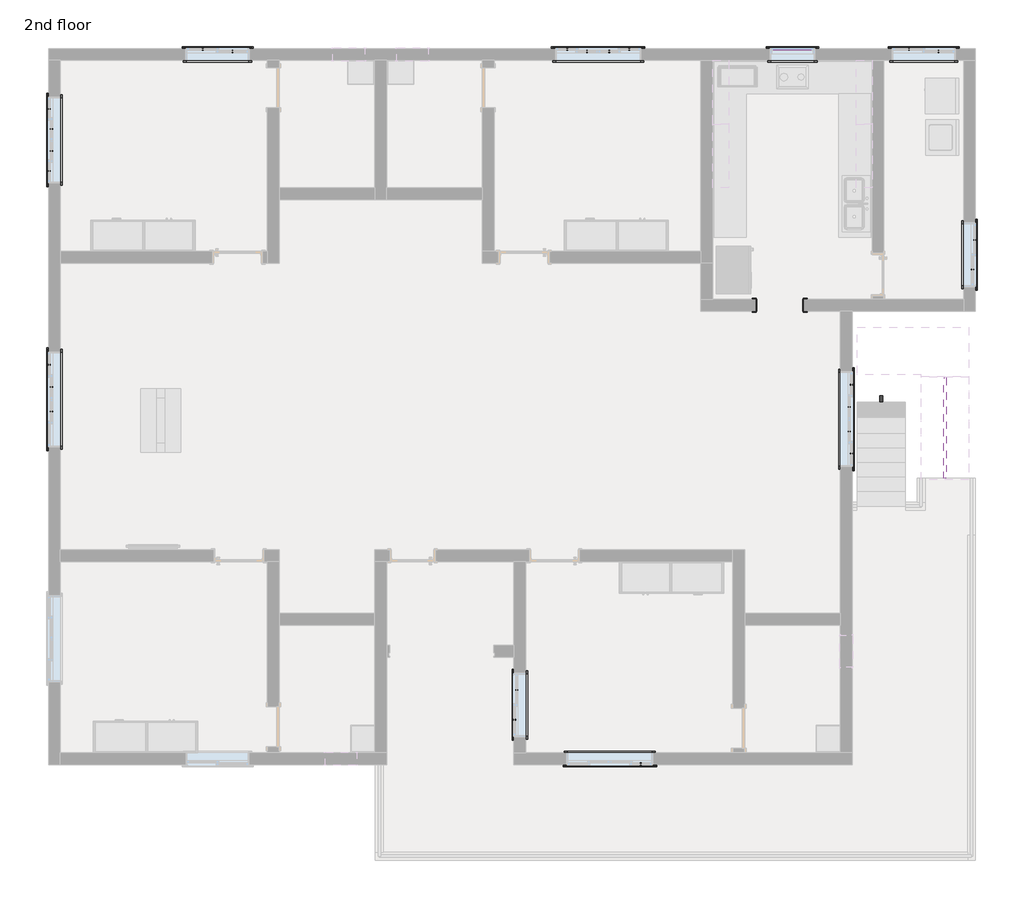
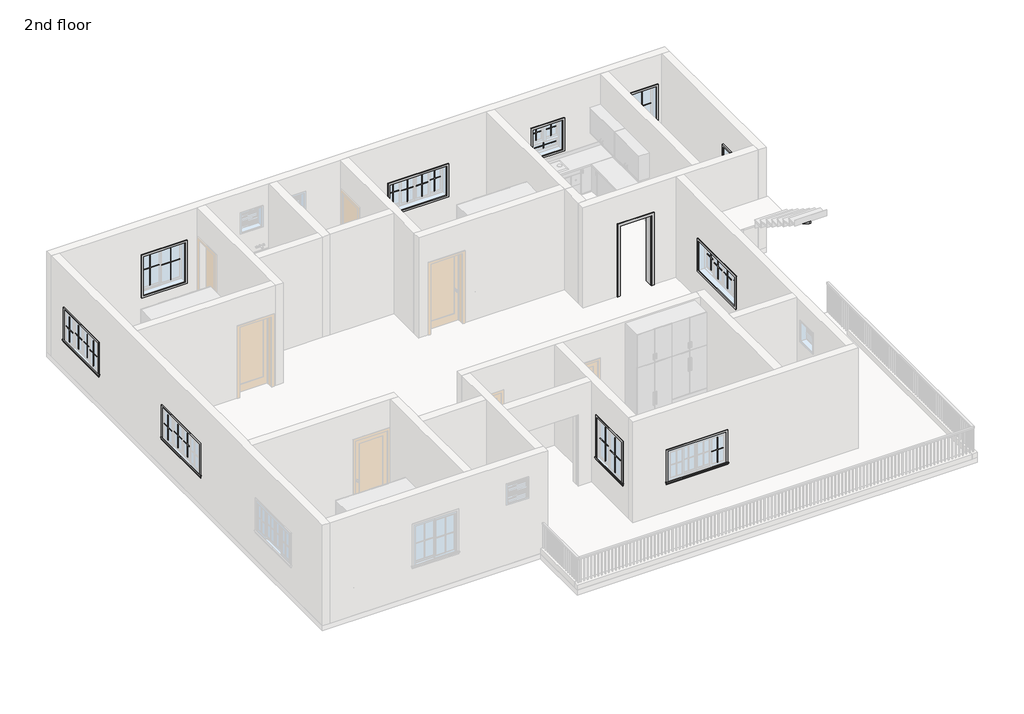
# One storey, part 4 of 4: 48 proxies, 2 members.
"""IFC4 building model written with IfcOpenShell, lengths in millimetres."""

from ifc_helpers import new_model, si_unit, frame, origin, place, context, project, spatial, polyline, outline, extrude, transform, mapped, element, save
from components import muntin_pattern_2x2_muntin_pattern_2x2_6186d23a, muntin_pattern_2x2_muntin_pattern_2x2_31a16349, muntin_pattern_2x2_muntin_pattern_2x2_cf37b409, muntin_pattern_2x2_muntin_pattern_2x2_78ce0566, muntin_pattern_2x2_muntin_pattern_2x2_27bf4e5b, muntin_pattern_2x2_muntin_pattern_2x2_8320156c, proxy_e9bf662a, trim_window_exterior_flat_with_sill_c3f87112, trim_window_exterior_flat_with_sill_3c945769, trim_window_exterior_flat_with_sill_7cfdd449, trim_window_exterior_flat_with_sill_41619996, trim_window_interior_flat_picture_frame_1c33fa8a, trim_window_interior_flat_picture_frame_0edfbaa2, trim_window_interior_flat_picture_frame_f1e0b15b, trim_window_interior_flat_picture_frame_51c85655

model = new_model("IFC4")

# Units and contexts
model_context = context("Model", 3, world=origin())
ifc_project = project(units=[si_unit("LENGTHUNIT", "METRE", prefix="MILLI")], contexts=[model_context])

# Site, building, storey
site = spatial("IfcSite", under=ifc_project)
building = spatial("IfcBuilding", under=site)
storey = spatial("IfcBuildingStorey", under=building, Name="2nd floor", Elevation=7010.4)

# Proxies
placement = place(None, origin())
muntin_pattern_2x2_muntin_pattern_2x2_shape = muntin_pattern_2x2_muntin_pattern_2x2_6186d23a(model_context)
element("IfcBuildingElementProxy", 1, Name="Muntin Pattern_2x2 : Muntin Pattern_2x2", ObjectType="Muntin Pattern_2x2 : Muntin Pattern_2x2", at=placement, inside=storey, context=model_context, shape_type="MappedRepresentation", body=[
    mapped(muntin_pattern_2x2_muntin_pattern_2x2_shape, transform((1905.0010838, 7064.4410813, 8007.35), x_axis=(1.0, 0.0, 0.0), y_axis=(0.0, 1.0, 0.0), z_axis=(0.0, 0.0, 1.0))),
])
element("IfcBuildingElementProxy", 2, Name="Muntin Pattern_2x2 : Muntin Pattern_2x2", ObjectType="Muntin Pattern_2x2 : Muntin Pattern_2x2", at=placement, inside=storey, context=model_context, shape_type="MappedRepresentation", body=[
    mapped(muntin_pattern_2x2_muntin_pattern_2x2_shape, transform((2286.0010838, 7019.9910813, 8007.35), x_axis=(1.0, 0.0, 0.0), y_axis=(0.0, 1.0, 0.0), z_axis=(0.0, 0.0, 1.0))),
])
element("IfcBuildingElementProxy", 3, Name="Muntin Pattern_2x2 : Muntin Pattern_2x2", ObjectType="Muntin Pattern_2x2 : Muntin Pattern_2x2", at=placement, inside=storey, context=model_context, shape_type="MappedRepresentation", body=[
    mapped(muntin_pattern_2x2_muntin_pattern_2x2_shape, transform((2711.4510838, 7019.9910813, 8007.35), x_axis=(1.0, 0.0, 0.0), y_axis=(0.0, 1.0, 0.0), z_axis=(0.0, 0.0, 1.0))),
])
element("IfcBuildingElementProxy", 4, Name="Muntin Pattern_2x2 : Muntin Pattern_2x2", ObjectType="Muntin Pattern_2x2 : Muntin Pattern_2x2", at=placement, inside=storey, context=model_context, shape_type="MappedRepresentation", body=[
    mapped(muntin_pattern_2x2_muntin_pattern_2x2_shape, transform((3092.4510838, 7064.4410813, 8007.35), x_axis=(1.0, 0.0, 0.0), y_axis=(0.0, 1.0, 0.0), z_axis=(0.0, 0.0, 1.0))),
])
element("IfcBuildingElementProxy", 5, Name="Muntin Pattern_2x2 : Muntin Pattern_2x2", ObjectType="Muntin Pattern_2x2 : Muntin Pattern_2x2", at=placement, inside=storey, context=model_context, shape_type="MappedRepresentation", body=[
    mapped(muntin_pattern_2x2_muntin_pattern_2x2_shape, transform((3314.7010838, -6632.5089187, 8007.35), x_axis=(-1.0, 0.0, 0.0), y_axis=(0.0, -1.0, 0.0), z_axis=(0.0, 0.0, 1.0))),
])
element("IfcBuildingElementProxy", 6, Name="Muntin Pattern_2x2 : Muntin Pattern_2x2", ObjectType="Muntin Pattern_2x2 : Muntin Pattern_2x2", at=placement, inside=storey, context=model_context, shape_type="MappedRepresentation", body=[
    mapped(muntin_pattern_2x2_muntin_pattern_2x2_shape, transform((-8020.0489162, 4727.6410813, 8007.35), x_axis=(0.0, 1.0, 0.0), y_axis=(-1.0, 0.0, 0.0), z_axis=(0.0, 0.0, 1.0))),
])
element("IfcBuildingElementProxy", 7, Name="Muntin Pattern_2x2 : Muntin Pattern_2x2", ObjectType="Muntin Pattern_2x2 : Muntin Pattern_2x2", at=placement, inside=storey, context=model_context, shape_type="MappedRepresentation", body=[
    mapped(muntin_pattern_2x2_muntin_pattern_2x2_shape, transform((-7975.5989162, 5108.6410813, 8007.35), x_axis=(0.0, 1.0, 0.0), y_axis=(-1.0, 0.0, 0.0), z_axis=(0.0, 0.0, 1.0))),
])
element("IfcBuildingElementProxy", 8, Name="Muntin Pattern_2x2 : Muntin Pattern_2x2", ObjectType="Muntin Pattern_2x2 : Muntin Pattern_2x2", at=placement, inside=storey, context=model_context, shape_type="MappedRepresentation", body=[
    mapped(muntin_pattern_2x2_muntin_pattern_2x2_shape, transform((-7975.5989162, 5534.0910813, 8007.35), x_axis=(0.0, 1.0, 0.0), y_axis=(-1.0, 0.0, 0.0), z_axis=(0.0, 0.0, 1.0))),
])
element("IfcBuildingElementProxy", 9, Name="Muntin Pattern_2x2 : Muntin Pattern_2x2", ObjectType="Muntin Pattern_2x2 : Muntin Pattern_2x2", at=placement, inside=storey, context=model_context, shape_type="MappedRepresentation", body=[
    mapped(muntin_pattern_2x2_muntin_pattern_2x2_shape, transform((-8020.0489162, 5915.0910813, 8007.35), x_axis=(0.0, 1.0, 0.0), y_axis=(-1.0, 0.0, 0.0), z_axis=(0.0, 0.0, 1.0))),
])
muntin_pattern_2x2_muntin_pattern_2x2_2_shape = muntin_pattern_2x2_muntin_pattern_2x2_31a16349(model_context)
element("IfcBuildingElementProxy", 10, Name="Muntin Pattern_2x2 : Muntin Pattern_2x2", ObjectType="Muntin Pattern_2x2 : Muntin Pattern_2x2", at=placement, inside=storey, context=model_context, shape_type="MappedRepresentation", body=[
    mapped(muntin_pattern_2x2_muntin_pattern_2x2_2_shape, transform((-7975.5989162, 120.7160813, 8007.35), x_axis=(0.0, 1.0, 0.0), y_axis=(-1.0, 0.0, 0.0), z_axis=(0.0, 0.0, 1.0))),
])
element("IfcBuildingElementProxy", 11, Name="Muntin Pattern_2x2 : Muntin Pattern_2x2", ObjectType="Muntin Pattern_2x2 : Muntin Pattern_2x2", at=placement, inside=storey, context=model_context, shape_type="MappedRepresentation", body=[
    mapped(muntin_pattern_2x2_muntin_pattern_2x2_2_shape, transform((-7975.5989162, 590.6160813, 8007.35), x_axis=(0.0, 1.0, 0.0), y_axis=(-1.0, 0.0, 0.0), z_axis=(0.0, 0.0, 1.0))),
])
element("IfcBuildingElementProxy", 12, Name="Muntin Pattern_2x2 : Muntin Pattern_2x2", ObjectType="Muntin Pattern_2x2 : Muntin Pattern_2x2", at=placement, inside=storey, context=model_context, shape_type="MappedRepresentation", body=[
    mapped(muntin_pattern_2x2_muntin_pattern_2x2_2_shape, transform((-8020.0489162, 1016.0660813, 8007.35), x_axis=(0.0, 1.0, 0.0), y_axis=(-1.0, 0.0, 0.0), z_axis=(0.0, 0.0, 1.0))),
])
element("IfcBuildingElementProxy", 13, Name="Muntin Pattern_2x2 : Muntin Pattern_2x2", ObjectType="Muntin Pattern_2x2 : Muntin Pattern_2x2", at=placement, inside=storey, context=model_context, shape_type="MappedRepresentation", body=[
    mapped(muntin_pattern_2x2_muntin_pattern_2x2_2_shape, transform((7353.3010838, 635.0660813, 8007.35), x_axis=(0.0, -1.0, 0.0), y_axis=(1.0, 0.0, 0.0), z_axis=(0.0, 0.0, 1.0))),
])
element("IfcBuildingElementProxy", 14, Name="Muntin Pattern_2x2 : Muntin Pattern_2x2", ObjectType="Muntin Pattern_2x2 : Muntin Pattern_2x2", at=placement, inside=storey, context=model_context, shape_type="MappedRepresentation", body=[
    mapped(muntin_pattern_2x2_muntin_pattern_2x2_2_shape, transform((7308.8510838, 209.6160813, 8007.35), x_axis=(0.0, -1.0, 0.0), y_axis=(1.0, 0.0, 0.0), z_axis=(0.0, 0.0, 1.0))),
])
element("IfcBuildingElementProxy", 15, Name="Muntin Pattern_2x2 : Muntin Pattern_2x2", ObjectType="Muntin Pattern_2x2 : Muntin Pattern_2x2", at=placement, inside=storey, context=model_context, shape_type="MappedRepresentation", body=[
    mapped(muntin_pattern_2x2_muntin_pattern_2x2_2_shape, transform((7308.8510838, -260.2839187, 8007.35), x_axis=(0.0, -1.0, 0.0), y_axis=(1.0, 0.0, 0.0), z_axis=(0.0, 0.0, 1.0))),
])
element("IfcBuildingElementProxy", 16, Name="Muntin Pattern_2x2 : Muntin Pattern_2x2", ObjectType="Muntin Pattern_2x2 : Muntin Pattern_2x2", at=placement, inside=storey, context=model_context, shape_type="MappedRepresentation", body=[
    mapped(muntin_pattern_2x2_muntin_pattern_2x2_2_shape, transform((7353.3010838, -685.7339187, 8007.35), x_axis=(0.0, -1.0, 0.0), y_axis=(1.0, 0.0, 0.0), z_axis=(0.0, 0.0, 1.0))),
])
muntin_pattern_2x2_muntin_pattern_2x2_3_shape = muntin_pattern_2x2_muntin_pattern_2x2_cf37b409(model_context)
element("IfcBuildingElementProxy", 17, Name="Muntin Pattern_2x2 : Muntin Pattern_2x2", ObjectType="Muntin Pattern_2x2 : Muntin Pattern_2x2", at=placement, inside=storey, context=model_context, shape_type="MappedRepresentation", body=[
    mapped(muntin_pattern_2x2_muntin_pattern_2x2_3_shape, transform((939.8010838, -5214.8714187, 8007.35), x_axis=(0.0, 1.0, 0.0), y_axis=(-1.0, 0.0, 0.0), z_axis=(0.0, 0.0, 1.0))),
])
element("IfcBuildingElementProxy", 18, Name="Muntin Pattern_2x2 : Muntin Pattern_2x2", ObjectType="Muntin Pattern_2x2 : Muntin Pattern_2x2", at=placement, inside=storey, context=model_context, shape_type="MappedRepresentation", body=[
    mapped(muntin_pattern_2x2_muntin_pattern_2x2_3_shape, transform((895.3510838, -5783.1964187, 8007.35), x_axis=(0.0, 1.0, 0.0), y_axis=(-1.0, 0.0, 0.0), z_axis=(0.0, 0.0, 1.0))),
])
element("IfcBuildingElementProxy", 19, Name="Muntin Pattern_2x2 : Muntin Pattern_2x2", ObjectType="Muntin Pattern_2x2 : Muntin Pattern_2x2", at=placement, inside=storey, context=model_context, shape_type="MappedRepresentation", body=[
    mapped(muntin_pattern_2x2_muntin_pattern_2x2_3_shape, transform((9018.5885838, 7019.9910813, 8007.35), x_axis=(1.0, 0.0, 0.0), y_axis=(0.0, 1.0, 0.0), z_axis=(0.0, 0.0, 1.0))),
])
element("IfcBuildingElementProxy", 20, Name="Muntin Pattern_2x2 : Muntin Pattern_2x2", ObjectType="Muntin Pattern_2x2 : Muntin Pattern_2x2", at=placement, inside=storey, context=model_context, shape_type="MappedRepresentation", body=[
    mapped(muntin_pattern_2x2_muntin_pattern_2x2_3_shape, transform((8450.2635838, 7064.4410813, 8007.35), x_axis=(1.0, 0.0, 0.0), y_axis=(0.0, 1.0, 0.0), z_axis=(0.0, 0.0, 1.0))),
])
element("IfcBuildingElementProxy", 21, Name="Muntin Pattern_2x2 : Muntin Pattern_2x2", ObjectType="Muntin Pattern_2x2 : Muntin Pattern_2x2", at=placement, inside=storey, context=model_context, shape_type="MappedRepresentation", body=[
    mapped(muntin_pattern_2x2_muntin_pattern_2x2_3_shape, transform((9671.0510838, 2840.1035813, 8007.35), x_axis=(0.0, -1.0, 0.0), y_axis=(1.0, 0.0, 0.0), z_axis=(0.0, 0.0, 1.0))),
])
element("IfcBuildingElementProxy", 22, Name="Muntin Pattern_2x2 : Muntin Pattern_2x2", ObjectType="Muntin Pattern_2x2 : Muntin Pattern_2x2", at=placement, inside=storey, context=model_context, shape_type="MappedRepresentation", body=[
    mapped(muntin_pattern_2x2_muntin_pattern_2x2_3_shape, transform((9715.5010838, 3408.4285813, 8007.35), x_axis=(0.0, -1.0, 0.0), y_axis=(1.0, 0.0, 0.0), z_axis=(0.0, 0.0, 1.0))),
])
element("IfcBuildingElementProxy", 23, Name="Muntin Pattern_2x2 : Muntin Pattern_2x2", ObjectType="Muntin Pattern_2x2 : Muntin Pattern_2x2", at=placement, inside=storey, context=model_context, shape_type="MappedRepresentation", body=[
    mapped(muntin_pattern_2x2_muntin_pattern_2x2_3_shape, transform((-4506.9114162, 7019.9910813, 8007.35), x_axis=(1.0, 0.0, 0.0), y_axis=(0.0, 1.0, 0.0), z_axis=(0.0, 0.0, 1.0))),
])
element("IfcBuildingElementProxy", 24, Name="Muntin Pattern_2x2 : Muntin Pattern_2x2", ObjectType="Muntin Pattern_2x2 : Muntin Pattern_2x2", at=placement, inside=storey, context=model_context, shape_type="MappedRepresentation", body=[
    mapped(muntin_pattern_2x2_muntin_pattern_2x2_3_shape, transform((-5075.2364162, 7064.4410813, 8007.35), x_axis=(1.0, 0.0, 0.0), y_axis=(0.0, 1.0, 0.0), z_axis=(0.0, 0.0, 1.0))),
])
muntin_pattern_2x2_muntin_pattern_2x2_4_shape = muntin_pattern_2x2_muntin_pattern_2x2_78ce0566(model_context)
element("IfcBuildingElementProxy", 25, Name="Muntin Pattern_2x2 : Muntin Pattern_2x2", ObjectType="Muntin Pattern_2x2 : Muntin Pattern_2x2", at=placement, inside=storey, context=model_context, shape_type="MappedRepresentation", body=[
    mapped(muntin_pattern_2x2_muntin_pattern_2x2_4_shape, transform((6005.5135838, 7064.4410813, 8528.05), x_axis=(1.0, 0.0, 0.0), y_axis=(0.0, 1.0, 0.0), z_axis=(0.0, 0.0, 1.0))),
])
muntin_pattern_2x2_muntin_pattern_2x2_5_shape = muntin_pattern_2x2_muntin_pattern_2x2_27bf4e5b(model_context)
element("IfcBuildingElementProxy", 26, Name="Muntin Pattern_2x2 : Muntin Pattern_2x2", ObjectType="Muntin Pattern_2x2 : Muntin Pattern_2x2", at=placement, inside=storey, context=model_context, shape_type="MappedRepresentation", body=[
    mapped(muntin_pattern_2x2_muntin_pattern_2x2_5_shape, transform((6434.1385838, 7064.4410813, 8528.05), x_axis=(-1.0, 0.0, 0.0), y_axis=(0.0, -1.0, 0.0), z_axis=(0.0, 0.0, 1.0))),
])
muntin_pattern_2x2_muntin_pattern_2x2_6_shape = muntin_pattern_2x2_muntin_pattern_2x2_8320156c(model_context)
element("IfcBuildingElementProxy", 27, Name="Muntin Pattern_2x2 : Muntin Pattern_2x2", ObjectType="Muntin Pattern_2x2 : Muntin Pattern_2x2", at=placement, inside=storey, context=model_context, shape_type="MappedRepresentation", body=[
    mapped(muntin_pattern_2x2_muntin_pattern_2x2_6_shape, transform((6219.8260838, 7064.4410813, 8223.25), x_axis=(-1.0, 0.0, 0.0), y_axis=(0.0, -1.0, 0.0), z_axis=(0.0, 0.0, 1.0))),
])
proxy_shape = proxy_e9bf662a(model_context)
element("IfcBuildingElementProxy", 28, Name="Passage Opening-Cased : 36\" x 84\"", ObjectType="Passage Opening-Cased : 36\" x 84\"", at=placement, inside=storey, context=model_context, shape_type="MappedRepresentation", body=[
    mapped(proxy_shape, transform((5970.337427, 2159.0660813, 7010.4), x_axis=(-1.0, 0.0, 0.0), y_axis=(0.0, -1.0, 0.0), z_axis=(0.0, 0.0, 1.0))),
])
trim_window_exterior_flat_with_sill_shape = trim_window_exterior_flat_with_sill_c3f87112(model_context)
element("IfcBuildingElementProxy", 29, Name="Trim-Window-Exterior-Flat : with Sill", ObjectType="Trim-Window-Exterior-Flat : with Sill", at=placement, inside=storey, context=model_context, shape_type="MappedRepresentation", body=[
    mapped(trim_window_exterior_flat_with_sill_shape, transform((2498.7260838, 7073.9660813, 8839.2), x_axis=(-1.0, 0.0, 0.0), y_axis=(0.0, 0.0, 1.0), z_axis=(0.0, 1.0, 0.0))),
])
element("IfcBuildingElementProxy", 30, Name="Trim-Window-Exterior-Flat : with Sill", ObjectType="Trim-Window-Exterior-Flat : with Sill", at=placement, inside=storey, context=model_context, shape_type="MappedRepresentation", body=[
    mapped(trim_window_exterior_flat_with_sill_shape, transform((2720.9760838, -6642.0339187, 8839.2), x_axis=(1.0, 0.0, 0.0), y_axis=(0.0, 0.0, 1.0), z_axis=(0.0, -1.0, 0.0))),
])
element("IfcBuildingElementProxy", 31, Name="Trim-Window-Exterior-Flat : with Sill", ObjectType="Trim-Window-Exterior-Flat : with Sill", at=placement, inside=storey, context=model_context, shape_type="MappedRepresentation", body=[
    mapped(trim_window_exterior_flat_with_sill_shape, transform((-8029.5739162, 5321.3660813, 8839.2), x_axis=(0.0, -1.0, 0.0), y_axis=(0.0, 0.0, 1.0), z_axis=(-1.0, 0.0, 0.0))),
])
trim_window_exterior_flat_with_sill_2_shape = trim_window_exterior_flat_with_sill_3c945769(model_context)
element("IfcBuildingElementProxy", 32, Name="Trim-Window-Exterior-Flat : with Sill", ObjectType="Trim-Window-Exterior-Flat : with Sill", at=placement, inside=storey, context=model_context, shape_type="MappedRepresentation", body=[
    mapped(trim_window_exterior_flat_with_sill_2_shape, transform((-8029.5739162, 355.6660813, 8839.2), x_axis=(0.0, -1.0, 0.0), y_axis=(0.0, 0.0, 1.0), z_axis=(-1.0, 0.0, 0.0))),
])
element("IfcBuildingElementProxy", 33, Name="Trim-Window-Exterior-Flat : with Sill", ObjectType="Trim-Window-Exterior-Flat : with Sill", at=placement, inside=storey, context=model_context, shape_type="MappedRepresentation", body=[
    mapped(trim_window_exterior_flat_with_sill_2_shape, transform((7362.8260838, -25.3339187, 8839.2), x_axis=(0.0, 1.0, 0.0), y_axis=(0.0, 0.0, 1.0), z_axis=(1.0, 0.0, 0.0))),
])
trim_window_exterior_flat_with_sill_3_shape = trim_window_exterior_flat_with_sill_7cfdd449(model_context)
element("IfcBuildingElementProxy", 34, Name="Trim-Window-Exterior-Flat : with Sill", ObjectType="Trim-Window-Exterior-Flat : with Sill", at=placement, inside=storey, context=model_context, shape_type="MappedRepresentation", body=[
    mapped(trim_window_exterior_flat_with_sill_3_shape, transform((885.8260838, -5499.0339187, 9144.0), x_axis=(0.0, -1.0, 0.0), y_axis=(0.0, 0.0, 1.0), z_axis=(-1.0, 0.0, 0.0))),
])
element("IfcBuildingElementProxy", 35, Name="Trim-Window-Exterior-Flat : with Sill", ObjectType="Trim-Window-Exterior-Flat : with Sill", at=placement, inside=storey, context=model_context, shape_type="MappedRepresentation", body=[
    mapped(trim_window_exterior_flat_with_sill_3_shape, transform((8734.4260838, 7073.9660813, 9144.0), x_axis=(-1.0, 0.0, 0.0), y_axis=(0.0, 0.0, 1.0), z_axis=(0.0, 1.0, 0.0))),
])
element("IfcBuildingElementProxy", 36, Name="Trim-Window-Exterior-Flat : with Sill", ObjectType="Trim-Window-Exterior-Flat : with Sill", at=placement, inside=storey, context=model_context, shape_type="MappedRepresentation", body=[
    mapped(trim_window_exterior_flat_with_sill_3_shape, transform((9725.0260838, 3124.2660813, 9144.0), x_axis=(0.0, 1.0, 0.0), y_axis=(0.0, 0.0, 1.0), z_axis=(1.0, 0.0, 0.0))),
])
element("IfcBuildingElementProxy", 37, Name="Trim-Window-Exterior-Flat : with Sill", ObjectType="Trim-Window-Exterior-Flat : with Sill", at=placement, inside=storey, context=model_context, shape_type="MappedRepresentation", body=[
    mapped(trim_window_exterior_flat_with_sill_3_shape, transform((-4791.0739162, 7073.9660813, 9144.0), x_axis=(-1.0, 0.0, 0.0), y_axis=(0.0, 0.0, 1.0), z_axis=(0.0, 1.0, 0.0))),
])
trim_window_exterior_flat_with_sill_4_shape = trim_window_exterior_flat_with_sill_41619996(model_context)
element("IfcBuildingElementProxy", 38, Name="Trim-Window-Exterior-Flat : with Sill", ObjectType="Trim-Window-Exterior-Flat : with Sill", at=placement, inside=storey, context=model_context, shape_type="MappedRepresentation", body=[
    mapped(trim_window_exterior_flat_with_sill_4_shape, transform((6219.8260838, 7073.9660813, 9067.8), x_axis=(-1.0, 0.0, 0.0), y_axis=(0.0, 0.0, 1.0), z_axis=(0.0, 1.0, 0.0))),
])
trim_window_interior_flat_picture_frame_shape = trim_window_interior_flat_picture_frame_1c33fa8a(model_context)
element("IfcBuildingElementProxy", 39, Name="Trim-Window-Interior-Flat : Picture Frame", ObjectType="Trim-Window-Interior-Flat : Picture Frame", at=placement, inside=storey, context=model_context, shape_type="MappedRepresentation", body=[
    mapped(trim_window_interior_flat_picture_frame_shape, transform((2498.7260838, 6845.3660813, 8839.2), x_axis=(1.0, 0.0, 0.0), y_axis=(0.0, 0.0, 1.0), z_axis=(0.0, -1.0, 0.0))),
])
element("IfcBuildingElementProxy", 40, Name="Trim-Window-Interior-Flat : Picture Frame", ObjectType="Trim-Window-Interior-Flat : Picture Frame", at=placement, inside=storey, context=model_context, shape_type="MappedRepresentation", body=[
    mapped(trim_window_interior_flat_picture_frame_shape, transform((2720.9760838, -6413.4339187, 8839.2), x_axis=(-1.0, 0.0, 0.0), y_axis=(0.0, 0.0, 1.0), z_axis=(0.0, 1.0, 0.0))),
])
element("IfcBuildingElementProxy", 41, Name="Trim-Window-Interior-Flat : Picture Frame", ObjectType="Trim-Window-Interior-Flat : Picture Frame", at=placement, inside=storey, context=model_context, shape_type="MappedRepresentation", body=[
    mapped(trim_window_interior_flat_picture_frame_shape, transform((-7800.9739162, 5321.3660813, 8839.2), x_axis=(0.0, 1.0, 0.0), y_axis=(0.0, 0.0, 1.0), z_axis=(1.0, 0.0, 0.0))),
])
trim_window_interior_flat_picture_frame_2_shape = trim_window_interior_flat_picture_frame_0edfbaa2(model_context)
element("IfcBuildingElementProxy", 42, Name="Trim-Window-Interior-Flat : Picture Frame", ObjectType="Trim-Window-Interior-Flat : Picture Frame", at=placement, inside=storey, context=model_context, shape_type="MappedRepresentation", body=[
    mapped(trim_window_interior_flat_picture_frame_2_shape, transform((-7800.9739162, 355.6660813, 8839.2), x_axis=(0.0, 1.0, 0.0), y_axis=(0.0, 0.0, 1.0), z_axis=(1.0, 0.0, 0.0))),
])
element("IfcBuildingElementProxy", 43, Name="Trim-Window-Interior-Flat : Picture Frame", ObjectType="Trim-Window-Interior-Flat : Picture Frame", at=placement, inside=storey, context=model_context, shape_type="MappedRepresentation", body=[
    mapped(trim_window_interior_flat_picture_frame_2_shape, transform((7134.2260838, -25.3339187, 8839.2), x_axis=(0.0, -1.0, 0.0), y_axis=(0.0, 0.0, 1.0), z_axis=(-1.0, 0.0, 0.0))),
])
trim_window_interior_flat_picture_frame_3_shape = trim_window_interior_flat_picture_frame_f1e0b15b(model_context)
element("IfcBuildingElementProxy", 44, Name="Trim-Window-Interior-Flat : Picture Frame", ObjectType="Trim-Window-Interior-Flat : Picture Frame", at=placement, inside=storey, context=model_context, shape_type="MappedRepresentation", body=[
    mapped(trim_window_interior_flat_picture_frame_3_shape, transform((1114.4260838, -5499.0339187, 9144.0), x_axis=(0.0, 1.0, 0.0), y_axis=(0.0, 0.0, 1.0), z_axis=(1.0, 0.0, 0.0))),
])
element("IfcBuildingElementProxy", 45, Name="Trim-Window-Interior-Flat : Picture Frame", ObjectType="Trim-Window-Interior-Flat : Picture Frame", at=placement, inside=storey, context=model_context, shape_type="MappedRepresentation", body=[
    mapped(trim_window_interior_flat_picture_frame_3_shape, transform((8734.4260838, 6845.3660813, 9144.0), x_axis=(1.0, 0.0, 0.0), y_axis=(0.0, 0.0, 1.0), z_axis=(0.0, -1.0, 0.0))),
])
element("IfcBuildingElementProxy", 46, Name="Trim-Window-Interior-Flat : Picture Frame", ObjectType="Trim-Window-Interior-Flat : Picture Frame", at=placement, inside=storey, context=model_context, shape_type="MappedRepresentation", body=[
    mapped(trim_window_interior_flat_picture_frame_3_shape, transform((9496.4260838, 3124.2660813, 9144.0), x_axis=(0.0, -1.0, 0.0), y_axis=(0.0, 0.0, 1.0), z_axis=(-1.0, 0.0, 0.0))),
])
element("IfcBuildingElementProxy", 47, Name="Trim-Window-Interior-Flat : Picture Frame", ObjectType="Trim-Window-Interior-Flat : Picture Frame", at=placement, inside=storey, context=model_context, shape_type="MappedRepresentation", body=[
    mapped(trim_window_interior_flat_picture_frame_3_shape, transform((-4791.0739162, 6845.3660813, 9144.0), x_axis=(1.0, 0.0, 0.0), y_axis=(0.0, 0.0, 1.0), z_axis=(0.0, -1.0, 0.0))),
])
trim_window_interior_flat_picture_frame_4_shape = trim_window_interior_flat_picture_frame_51c85655(model_context)
element("IfcBuildingElementProxy", 48, Name="Trim-Window-Interior-Flat : Picture Frame", ObjectType="Trim-Window-Interior-Flat : Picture Frame", at=placement, inside=storey, context=model_context, shape_type="MappedRepresentation", body=[
    mapped(trim_window_interior_flat_picture_frame_4_shape, transform((6219.8260838, 6845.3660813, 9067.8), x_axis=(1.0, 0.0, 0.0), y_axis=(0.0, 0.0, 1.0), z_axis=(0.0, -1.0, 0.0))),
])

# Members
element("IfcMember", 49, ObjectType="Carriage - 2\" Width", at=placement, inside=storey, context=model_context, shape_type="SweptSolid", body=[
    extrude(outline(polyline([(825.5660813, 8559.8), (825.5660813, 8464.3282995), (-1459.1783893, 7010.4), (-1657.2839187, 7010.4), (-1657.2839187, 7137.4), (-1377.8839187, 7137.4), (-1377.8839187, 7315.2), (-1098.4839187, 7315.2), (-1098.4839187, 7493.0), (-819.0839187, 7493.0), (-819.0839187, 7670.8), (-539.6839187, 7670.8), (-539.6839187, 7848.6), (-260.2839187, 7848.6), (-260.2839187, 8026.4), (19.1160813, 8026.4), (19.1160813, 8204.2), (298.5160813, 8204.2), (298.5160813, 8382.0), (577.9160813, 8382.0), (577.9160813, 8559.8), (825.5660813, 8559.8)])), frame((7896.2260838, 0.0, 0.0), z_axis=(1.0, 0.0, 0.0), x_axis=(0.0, 1.0, 0.0)), (0.0, 0.0, 1.0), 50.8),
])
element("IfcMember", 50, ObjectType="Carriage - 2\" Width", at=placement, inside=storey, context=model_context, shape_type="SweptSolid", body=[
    extrude(outline(polyline([(-1156.9972984, 9886.7282995), (-1156.9972984, 9982.2), (-909.3472984, 9982.2), (-909.3472984, 9804.4), (-629.9472984, 9804.4), (-629.9472984, 9626.6), (-350.5472984, 9626.6), (-350.5472984, 9448.8), (-71.1472984, 9448.8), (-71.1472984, 9271.0), (208.2527016, 9271.0), (208.2527016, 9093.2), (487.6527016, 9093.2), (487.6527016, 8915.4), (767.0527016, 8915.4), (767.0527016, 8662.332845), (-1156.9972984, 9886.7282995)])), frame((9115.4260838, 0.0, 0.0), z_axis=(1.0, 0.0, 0.0), x_axis=(0.0, 1.0, 0.0)), (0.0, 0.0, 1.0), 50.8),
])

save(model, "model.ifc")

# Revit data of these elements
# Type "Muntin Pattern_2x2 : Muntin Pattern_2x2"
#   Width [instance default] = 4' - 0"
#   Thickness = 0' - 0 1/2"
#   Height [instance default] = 4' - 0"
#   Distance = 0' - 0 3/4"
#   Interior Material [instance default] = none
#   Exterior Material [instance default] = none
#   Default Elevation = 0
# Type "Passage Opening-Cased : 36\" x 84\""
#   Height = 7' - 0"
#   Trim Thickness = 0' - 0 3/4"
#   Trim Width = 0' - 3"
#   Width = 3' - 0"
#   Frame Material = Door - Frame
#   Default Elevation = 0
# Type "Trim-Window-Exterior-Flat : with Sill"
#   Trim Width = 0' - 2 1/4"
#   Trim Thickness_Picture Frame = 0' - 1 1/4"
#   Trim Thickness_with Sill = 0' - 0 3/4"
#   Sill Thickness = 0' - 1 1/4"
#   Opening Width [instance default] = 2' - 0"
#   Opening Height [instance default] = 3' - 0"
#   Default Elevation = 4' - 0"
#   Sill = yes
#   Picture Frame = no
#   Trim Material [instance default] = none
# Type "Trim-Window-Interior-Flat : Picture Frame"
#   Trim Thickness_Picture Frame = 0' - 1 1/4"
#   Trim Width = 0' - 2 1/4"
#   Trim Thickness_with Sill = 0' - 0 3/4"
#   Sill Thickness = 0' - 1 1/4"
#   Opening Width [instance default] = 2' - 0"
#   Opening Height [instance default] = 3' - 0"
#   Default Elevation = 4' - 0"
#   Sill = no
#   Picture Frame = yes
#   Trim Material [instance default] = none
# Elements 1, 2, 3, 4, 5, 6, 7, 8, 9 (IfcBuildingElementProxy, "Muntin Pattern_2x2 : Muntin Pattern_2x2")
#   Width = 1' - 1 1/4"
#   Height = 2' - 6 1/4"
#   Interior Material = Wood - Stained
#   Exterior Material = Clad - White
#   Phase Created = New Construction
#   Materials on its faces: "Clad - White", "Wood - Stained"
# Elements 10, 11, 12, 13, 14, 15, 16 (IfcBuildingElementProxy, "Muntin Pattern_2x2 : Muntin Pattern_2x2")
#   Width = 1' - 3"
#   Height = 2' - 6 1/4"
#   Interior Material = Wood - Stained
#   Exterior Material = Clad - White
#   Phase Created = New Construction
#   Materials on its faces: "Clad - White", "Wood - Stained"
# Elements 17, 18, 19, 20, 21, 22, 23, 24 (IfcBuildingElementProxy, "Muntin Pattern_2x2 : Muntin Pattern_2x2")
#   Width = 1' - 8 5/8"
#   Height = 3' - 6 1/4"
#   Interior Material = Wood - Stained
#   Exterior Material = Clad - White
#   Phase Created = New Construction
#   Materials on its faces: "Clad - White", "Wood - Stained"
# Elements 25, 26 (IfcBuildingElementProxy, "Muntin Pattern_2x2 : Muntin Pattern_2x2")
#   Width = 0' - 11 5/8"
#   Height = 1' - 6 1/2"
#   Interior Material = Wood - Stained
#   Exterior Material = Clad - White
#   Phase Created = New Construction
#   Materials on its faces: "Clad - White", "Wood - Stained"
# Element 27 (IfcBuildingElementProxy, "Muntin Pattern_2x2 : Muntin Pattern_2x2")
#   Width = 2' - 4 1/2"
#   Height = 0' - 6 1/2"
#   Interior Material = Wood - Stained
#   Exterior Material = Clad - White
#   Phase Created = New Construction
#   Materials on its faces: "Clad - White", "Wood - Stained"
# Element 28 (IfcBuildingElementProxy, "Passage Opening-Cased : 36\" x 84\"")
#   Phase Created = New Construction
#   Materials on its faces: "Door - Frame"
# Elements 29, 30, 31 (IfcBuildingElementProxy, "Trim-Window-Exterior-Flat : with Sill")
#   Opening Width = 5' - 5"
#   Opening Height = 3' - 0"
#   Trim Material = Clad - White
#   Phase Created = New Construction
#   Materials on its faces: "Clad - White"
# Elements 32, 33 (IfcBuildingElementProxy, "Trim-Window-Exterior-Flat : with Sill")
#   Opening Width = 6' - 0"
#   Opening Height = 3' - 0"
#   Trim Material = Clad - White
#   Phase Created = New Construction
#   Materials on its faces: "Clad - White"
# Elements 34, 35, 36, 37 (IfcBuildingElementProxy, "Trim-Window-Exterior-Flat : with Sill")
#   Opening Width = 4' - 0"
#   Opening Height = 4' - 0"
#   Trim Material = Clad - White
#   Phase Created = New Construction
#   Materials on its faces: "Clad - White"
# Element 38 (IfcBuildingElementProxy, "Trim-Window-Exterior-Flat : with Sill")
#   Opening Width = 2' - 10"
#   Opening Height = 3' - 0"
#   Trim Material = Clad - White
#   Phase Created = New Construction
#   Materials on its faces: "Clad - White"
# Elements 39, 40, 41 (IfcBuildingElementProxy, "Trim-Window-Interior-Flat : Picture Frame")
#   Opening Width = 5' - 5"
#   Opening Height = 3' - 0"
#   Trim Material = Wood - Stained
#   Phase Created = New Construction
#   Materials on its faces: "Wood - Stained"
# Elements 42, 43 (IfcBuildingElementProxy, "Trim-Window-Interior-Flat : Picture Frame")
#   Opening Width = 6' - 0"
#   Opening Height = 3' - 0"
#   Trim Material = Wood - Stained
#   Phase Created = New Construction
#   Materials on its faces: "Wood - Stained"
# Elements 44, 45, 46, 47 (IfcBuildingElementProxy, "Trim-Window-Interior-Flat : Picture Frame")
#   Opening Width = 4' - 0"
#   Opening Height = 4' - 0"
#   Trim Material = Wood - Stained
#   Phase Created = New Construction
#   Materials on its faces: "Wood - Stained"
# Element 48 (IfcBuildingElementProxy, "Trim-Window-Interior-Flat : Picture Frame")
#   Opening Width = 2' - 10"
#   Opening Height = 3' - 0"
#   Trim Material = Wood - Stained
#   Phase Created = New Construction
#   Materials on its faces: "Wood - Stained"
# Elements 49, 50 (IfcMember, "Carriage - 2\" Width")
#   Phase Created = New Construction
# Materials
#   "Door - Frame": colour RGB 118 70 51, transparency 0, Cost = 0
#   "Clad - White": class "Wood", colour RGB 242 242 238, transparency 0, Cost = 0
#   "Wood - Stained": class "Wood", colour RGB 224 178 126, transparency 0, Cost = 0
